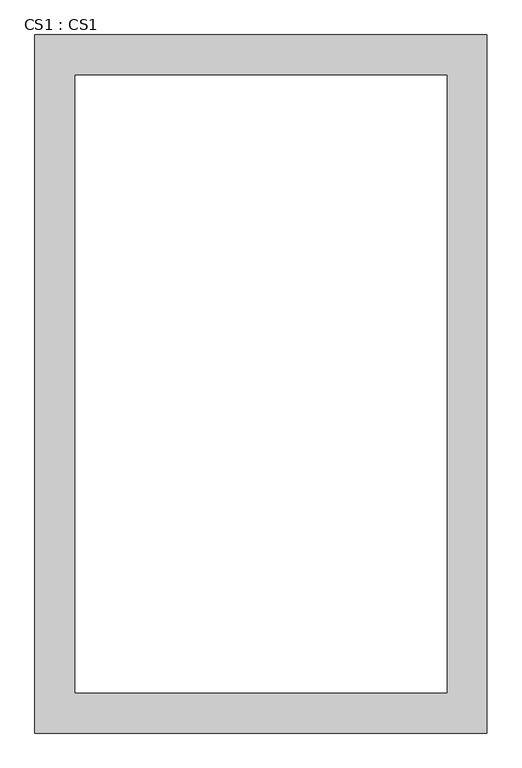
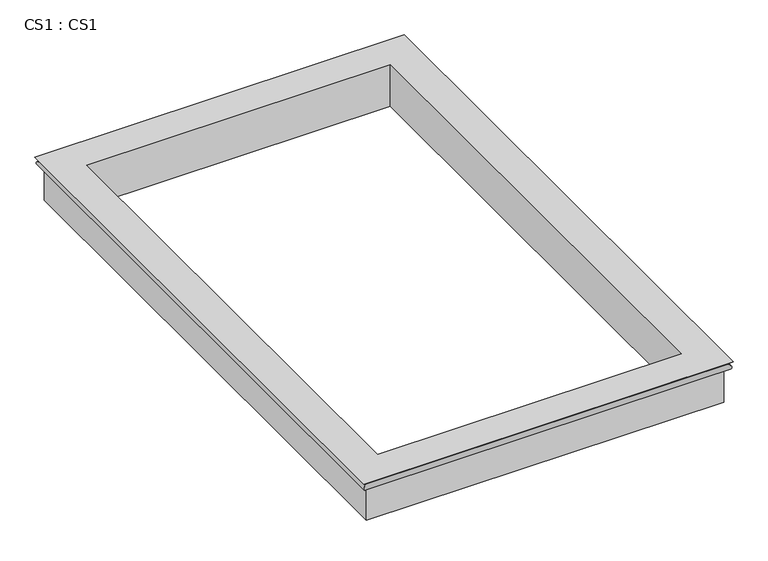
"""IFC4 building model written with IfcOpenShell, lengths in millimetres: furniture geometry, CS1 : CS1."""

from ifc_helpers import new_model, si_unit, frame, origin, place, context, project, spatial, ellipse_curve, source, transform, mapped, element, save
from ifc_brep_helpers import plane_surface, cylinder_surface, advanced_brep


def cs1_cs1_efe94d7d(model_context):
    return source(origin(), model_context, "Body", "AdvancedBrep", [
        advanced_brep(
        [(-8759.1005098, -16191.424748, 6779.203548), (-8778.822521, -16211.1467593, 6705.6), (-2581.222521, -16211.1467593, 6705.6), (-2600.9445323, -16191.424748, 6779.203548), (-2529.1024833, -16263.266797, 6851.0455969), (-8830.9425588, -16263.266797, 6851.0455969), (-8270.822521, -15703.1467593, 6096.0), (-8270.822521, -15703.1467593, 6851.0455969), (-3089.222521, -15703.1467593, 6851.0455969), (-3089.222521, -15703.1467593, 6096.0), (-8728.022521, -16160.3467593, 6705.6), (-8728.022521, -16160.3467593, 6096.0), (-2632.022521, -16160.3467593, 6096.0), (-2632.022521, -16160.3467593, 6705.6), (-2581.222521, -6587.7230207, 6705.6), (-2600.9445323, -6607.445032, 6779.203548), (-2529.1024833, -6535.602983, 6851.0455969), (-3089.222521, -7095.7230207, 6851.0455969), (-3089.222521, -7095.7230207, 6096.0), (-2632.022521, -6638.5230207, 6096.0), (-2632.022521, -6638.5230207, 6705.6), (-8778.822521, -6587.7230207, 6705.6), (-8759.1005098, -6607.445032, 6779.203548), (-8830.9425588, -6535.602983, 6851.0455969), (-8270.822521, -7095.7230207, 6851.0455969), (-8270.822521, -7095.7230207, 6096.0), (-8728.022521, -6638.5230207, 6096.0), (-8728.022521, -6638.5230207, 6705.6)],
        [
            (0, 1, ellipse_curve(frame((-8778.822521, -16211.1467593, 6745.0440225), z_axis=(0.707106781186546, -0.7071067811865489, 0.0), x_axis=(-0.707106781186549, -0.707106781186546, 0.0)), 55.7822715, 39.4440225)),
            (1, 2),
            (2, 3, ellipse_curve(frame((-2581.222521, -16211.1467593, 6745.0440225), z_axis=(-0.7071067811865489, -0.707106781186546, 0.0), x_axis=(-0.7071067811865461, 0.7071067811865488, 0.0)), 55.7822715, 39.4440225)),
            (3, 0),
            (3, 4),
            (4, 5),
            (5, 0),
            (6, 7),
            (7, 8),
            (8, 9),
            (9, 6),
            (10, 11),
            (11, 12),
            (12, 13),
            (13, 10),
            (2, 14),
            (14, 15, ellipse_curve(frame((-2581.222521, -6587.7230207, 6745.0440225), z_axis=(0.707106781186546, -0.7071067811865489, 0.0), x_axis=(-0.7071067811865488, -0.7071067811865461, 0.0)), 55.7822715, 39.4440225)),
            (15, 3),
            (15, 16),
            (16, 4),
            (8, 17),
            (17, 18),
            (18, 9),
            (12, 19),
            (19, 20),
            (20, 13),
            (14, 21),
            (21, 22, ellipse_curve(frame((-8778.822521, -6587.7230207, 6745.0440225), z_axis=(0.7071067811865489, 0.707106781186546, 0.0), x_axis=(0.7071067811865461, -0.7071067811865488, 0.0)), 55.7822715, 39.4440225)),
            (22, 15),
            (22, 23),
            (23, 16),
            (17, 24),
            (24, 25),
            (25, 18),
            (19, 26),
            (26, 27),
            (27, 20),
            (1, 21),
            (27, 10),
            (0, 22),
            (5, 23),
            (7, 24),
            (6, 25),
            (11, 26),
        ],
        [
            cylinder_surface(frame((-8728.022521, -16211.1467593, 6745.0440225), z_axis=(-1.0, 0.0, 0.0), x_axis=(0.0, 1.0, 0.0)), 39.4440225),
            plane_surface(frame((-8812.9820465, -16245.3062848, 6833.0850847), z_axis=(0.0, -0.7071067811865476, -0.7071067811865475), x_axis=(1.0, 0.0, 0.0))),
            plane_surface(frame((-8270.822521, -15703.1467593, 6851.0455969), z_axis=(0.0, 1.0, 0.0), x_axis=(1.0, 0.0, 0.0))),
            plane_surface(frame((-8728.022521, -16160.3467593, 6096.0), z_axis=(0.0, -1.0, 0.0), x_axis=(1.0, 0.0, 0.0))),
            cylinder_surface(frame((-2581.222521, -16160.3467593, 6745.0440225), z_axis=(0.0, -1.0, 0.0), x_axis=(-1.0, 0.0, 0.0)), 39.4440225),
            plane_surface(frame((-2547.0629955, -16245.3062848, 6833.0850847), z_axis=(0.7071067811865477, 0.0, -0.7071067811865475), x_axis=(0.0, 1.0, 0.0))),
            plane_surface(frame((-3089.222521, -15703.1467593, 6851.0455969), z_axis=(-1.0, 0.0, 0.0), x_axis=(0.0, 1.0, 0.0))),
            plane_surface(frame((-2632.022521, -16160.3467593, 6096.0), z_axis=(1.0, 0.0, 0.0), x_axis=(0.0, 1.0, 0.0))),
            cylinder_surface(frame((-2632.022521, -6587.7230207, 6745.0440225), z_axis=(1.0, 0.0, 0.0), x_axis=(0.0, -1.0, 0.0)), 39.4440225),
            plane_surface(frame((-2547.0629955, -6553.5634952, 6833.0850847), z_axis=(0.0, 0.7071067811865477, -0.7071067811865475), x_axis=(-1.0, 0.0, 0.0))),
            plane_surface(frame((-3089.222521, -7095.7230207, 6851.0455969), z_axis=(0.0, -1.0, 0.0), x_axis=(-1.0, 0.0, 0.0))),
            plane_surface(frame((-2632.022521, -6638.5230207, 6096.0), z_axis=(0.0, 1.0, 0.0), x_axis=(-1.0, 0.0, 0.0))),
            plane_surface(frame((-8728.022521, -6638.5230207, 6705.6), z_axis=(0.0, 0.0, -1.0), x_axis=(0.0, -1.0, 0.0))),
            cylinder_surface(frame((-8778.822521, -6638.5230207, 6745.0440225), z_axis=(0.0, 1.0, 0.0), x_axis=(1.0, 0.0, 0.0)), 39.4440225),
            plane_surface(frame((-8812.9820465, -6553.5634952, 6833.0850847), z_axis=(-0.7071067811865477, 0.0, -0.7071067811865474), x_axis=(0.0, -1.0, 0.0))),
            plane_surface(frame((-8729.3425588, -6637.202983, 6851.0455969), z_axis=(0.0, 0.0, 1.0), x_axis=(0.0, -1.0, 0.0))),
            plane_surface(frame((-8270.822521, -7095.7230207, 6851.0455969), z_axis=(1.0, 0.0, 0.0), x_axis=(0.0, -1.0, 0.0))),
            plane_surface(frame((-8270.822521, -7095.7230207, 6096.0), z_axis=(0.0, 0.0, -1.0), x_axis=(0.0, -1.0, 0.0))),
            plane_surface(frame((-8728.022521, -6638.5230207, 6096.0), z_axis=(-1.0, 0.0, 0.0), x_axis=(0.0, -1.0, 0.0))),
        ],
        [
            (0, [[1, 2, 3, 4]]),
            (1, [[-4, 5, 6, 7]]),
            (2, [[8, 9, 10, 11]]),
            (3, [[12, 13, 14, 15]]),
            (4, [[-3, 16, 17, 18]]),
            (5, [[-5, -18, 19, 20]]),
            (6, [[-10, 21, 22, 23]]),
            (7, [[-14, 24, 25, 26]]),
            (8, [[-17, 27, 28, 29]]),
            (9, [[-19, -29, 30, 31]]),
            (10, [[-22, 32, 33, 34]]),
            (11, [[-25, 35, 36, 37]]),
            (12, [[38, -27, -16, -2], [-26, -37, 39, -15]]),
            (13, [[-28, -38, -1, 40]]),
            (14, [[-30, -40, -7, 41]]),
            (15, [[-20, -31, -41, -6], [42, -32, -21, -9]]),
            (16, [[-33, -42, -8, 43]]),
            (17, [[44, -35, -24, -13], [-23, -34, -43, -11]]),
            (18, [[-36, -44, -12, -39]]),
        ],
    ),
    ])


if __name__ == "__main__":
    model = new_model("IFC4")
    model_context = context("Model", 3, world=origin())
    ifc_project = project(units=[si_unit("LENGTHUNIT", "METRE", prefix="MILLI")], contexts=[model_context])
    site = spatial("IfcSite", under=ifc_project)
    building = spatial("IfcBuilding", under=site)
    placement = place(None, origin())
    cs1_cs1_shape = cs1_cs1_efe94d7d(model_context)
    element("IfcFurniture", 1, ObjectType="CS1 : CS1", at=placement, inside=building, context=model_context, shape_type="MappedRepresentation", body=[
        mapped(cs1_cs1_shape, transform((0.0, 0.0, 0.0), x_axis=(1.0, 0.0, 0.0), y_axis=(0.0, 1.0, 0.0), z_axis=(0.0, 0.0, 1.0))),
    ])
    save(model, "model.ifc")

# Revit data of these elements
# Element 1 (IfcFurniture, "CS1 : CS1")
#   Materials on its faces: "Oak Flooring"
# Materials
#   "Oak Flooring": class "Wood", colour RGB 212 179 113, transparency 0, Description = "Quercus Rubra", Cost = 0
